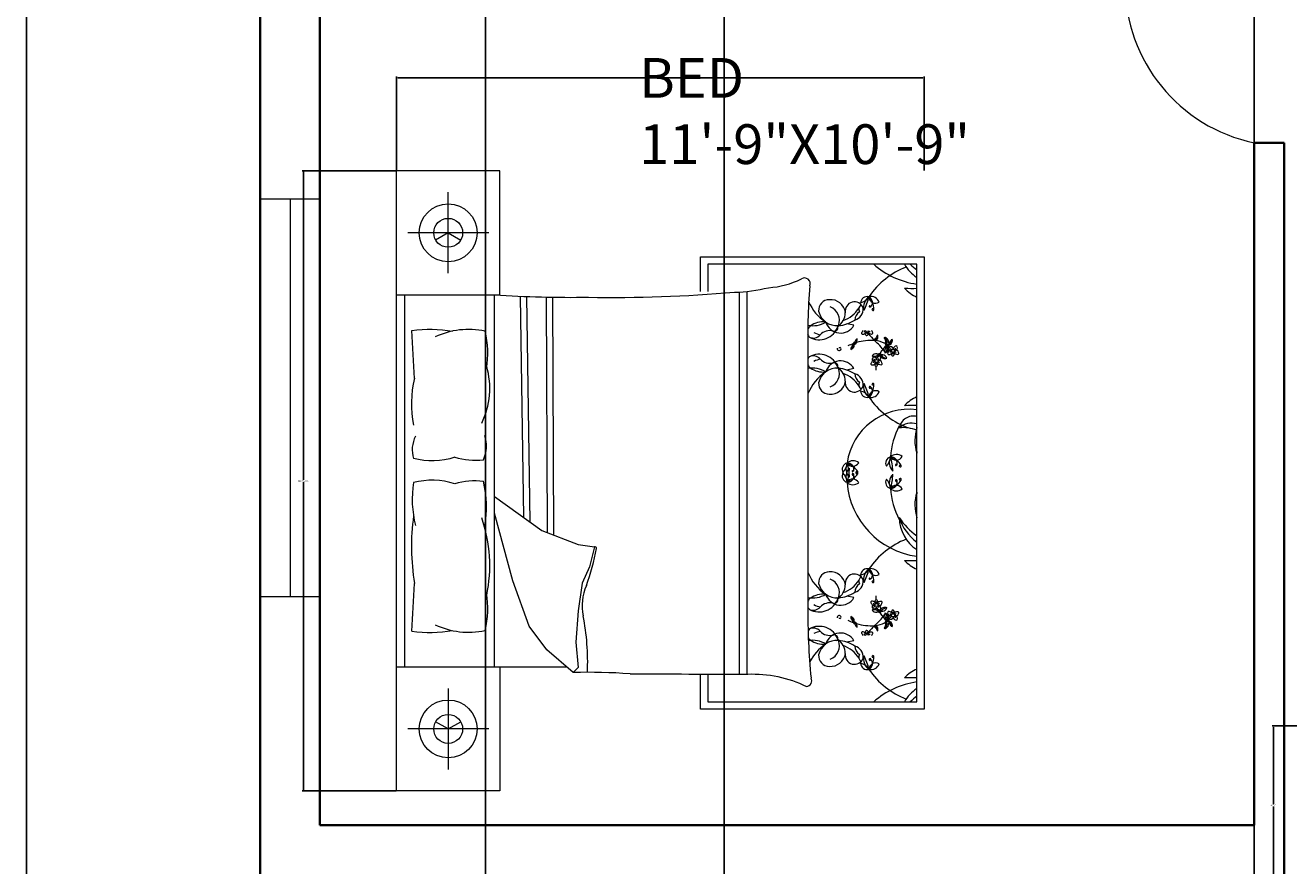
# Model space of a CAD drawing. Units: inches. Extents: x -59 to 444, y -680 to 63.
# Tile 4 of 9: x -59 to 132, y -270 to -143. Entities that reach past the tile are written whole.
import ezdxf

# ---------------------------------------------------------------- set-up
doc = ezdxf.new("R2010")
doc.units = ezdxf.units.IN
doc.header["$MEASUREMENT"] = 0
for name, color, linetype, lineweight in [('A-ANNO-DIMS', 2, 'Continuous', 18), ('A-AREA-IDEN', 7, 'Continuous', 18), ('A-DOOR', 3, 'Continuous', 18), ('A-FURN', 8, 'Continuous', 13), ('A-GLAZ', 4, 'Continuous', 18), ('A-WALL', 7, 'Continuous', 35)]:
    doc.layers.add(name, color=color, linetype=linetype, lineweight=lineweight)
doc.styles.get("Standard").update_dxf_attribs({"font": 'arial.ttf'})
doc.dimstyles.get("Standard").update_dxf_attribs({"dimtxt": 0.18, "dimasz": 0.18, "dimexe": 0.18, "dimexo": 0.0625, "dimgap": 0.09, "dimtad": 0, "dimtih": 1, "dimtoh": 1, "dimdec": 0, "dimzin": 0, "dimdsep": 46, "dimlunit": 3, "dimtxsty": 'Standard', "dimcen": 0.09, "dimadec": 0, "dimazin": 0, "dimtfac": 1, "dimtdec": 0, "dimtofl": 0, "dimtmove": 0, "dimatfit": 3, "dimfxl": 1, "dimtolj": 1, "dimtzin": 0, "dimarcsym": 0})

# ---------------------------------------------------------------- blocks, each defined once
blk = doc.blocks.new('BED-SET-80')
for p, q in [((0, 0), (0, 93.61)), ((7.8, 78.14), (7.8, 90.37)), ((13.92, 84.25), (1.69, 84.25)), ((45.89, 75.41), (45.89, 80.6)), ((45.89, 80.6), (79.61, 80.6)), ((79.61, 80.6), (79.61, 12.36)), ((46.97, 79.52), (46.97, 75.39)), ((78.53, 79.52), (46.97, 79.52)), ((78.53, 13.44), (78.53, 79.52)), ((1.2, 74.89), (1.2, 18.72)), ((14.79, 18.72), (14.79, 74.89)), ((18.68, 74.64), (19.15, 41.31)), ((19.64, 74.6), (20.12, 40.61)), ((22.59, 74.55), (22.73, 39.01)), ((23.55, 74.56), (23.7, 38.64)), ((51.73, 75.32), (51.73, 17.64)), ((52.89, 75.4), (52.89, 17.64)), ((69.04, 70.29), (67.98, 70.5)), ((62.09, 65.81), (62.09, 27.8)), ((69.04, 63.75), (67.98, 63.54)), ((14.79, 44.44), (21.93, 39.31)), ((17.58, 31.73), (14.79, 41.93)), ((21.93, 39.31), (27.43, 37.22)), ((27.43, 37.22), (29.89, 36.85)), ((29.89, 36.85), (29.13, 33.81)), ((29.13, 33.81), (28, 31.35)), ((20.04, 24.9), (17.58, 31.73)), ((28, 31.35), (27.43, 27.18)), ((69.04, 29.21), (67.98, 29.42)), ((27.43, 27.18), (27.05, 22.44)), ((22.69, 21.3), (20.04, 24.9)), ((26.67, 17.88), (22.69, 21.3)), ((27.05, 22.44), (27.43, 18.64)), ((69.04, 22.67), (67.98, 22.46)), ((0, 18.72), (25.69, 18.72)), ((27.43, 18.64), (26.67, 17.88)), ((45.89, 12.36), (45.89, 17.65)), ((46.97, 17.65), (46.97, 13.44)), ((7.8, 15.48), (7.8, 3.25)), ((46.97, 13.44), (78.53, 13.44)), ((79.61, 12.36), (45.89, 12.36)), ((13.92, 9.36), (1.69, 9.36))]:
    blk.add_line(p, q)
for points in [[(0, 74.89), (15.6, 74.89), (15.6, 93.61), (0, 93.61)], [(7.8, 84.25), (5.91, 83.16)], [(7.8, 84.25), (9.69, 83.16)], [(15.6, 18.72), (15.6, 0), (0, 0)], [(7.8, 9.36), (5.91, 10.45)], [(7.8, 9.36), (9.69, 10.45)]]:
    blk.add_lwpolyline(points)
for points in [[(50.99, 75.29, 0.056112), (56.14, 75.97, 0.095341), (61.1, 77.28)], [(2.33, 69.51, -0.074897), (8.45, 69.4, 0.472817)], [(8.79, 50.37, -0.14099), (2.55, 50.18, -0.235245)], [(8.79, 46.37, 0.14099), (2.55, 46.55, 0.235245)], [(2.33, 24.1, 0.074897), (8.45, 24.21, -0.472817)], [(35.24, 17.69, 0.001242), (53, 17.64, -0.127202), (61.86, 15.77)]]:
    blk.add_lwpolyline(points, format="xyb")
for centre, radius in [((7.8, 84.25), 4.37), ((7.8, 84.25), 2.18), ((72.43, 64.89), 0.238), ((74.94, 66.44), 0.238), ((72.43, 28.07), 0.238), ((74.94, 26.51), 0.238), ((7.8, 9.36), 4.37), ((7.8, 9.36), 2.18)]:
    blk.add_circle(centre, radius)
for centre, radius, start, end in [((81.38, 67.71), 12.22, 111.4092, 145.6135), ((80.17, 88.62), 12.22, 228.1144, 262.255), ((81.81, 82.49), 5.96, 209.8884, 236.5383), ((82.92, 84.63), 7.42, 223.5186, 233.6964), ((61.58, 76.58), 0.853, 336.5219, 123.8264), ((26.23, 242.71), 168.2, 266.1, 270.9282), ((32.35, 293.91), 219.42, 269.1145, 274.8735), ((153.14, 68.68), 91.09, 175.2402, 181.8035), ((71.05, 73.62), 1.01, 76.272, 177.0484), ((69.51, 75.7), 2.09, 284.7031, 328.6173), ((72.42, 73.04), 1.93, 125.7657, 194.5347), ((62.95, 76.46), 8.55, 332.8176, 347.4827), ((71.58, 73.28), 1.36, 20.9613, 102.2885), ((72.31, 74.64), 1.02, 181.7131, 301.5367), ((68.97, 72.57), 3.09, 2.0648, 41.1598), ((70.83, 73.72), 1, 316.2238, 62.3173), ((80.43, 79.15), 4.97, 221.0454, 247.4453), ((77.76, 92.77), 16.91, 266.3481, 272.5919), ((68.68, 76.7), 7.09, 203.6453, 236.3329), ((65.28, 72.57), 1.58, 88.9462, 185.5144), ((65.51, 71.92), 2.24, 7.1143, 95.0551), ((64.66, 71.04), 2.17, 338.5779, 68.4181), ((66.02, 75.22), 4.42, 288.2955, 328.7386), ((69.11, 72.43), 1.4, 19.1312, 189.736), ((68.69, 72.77), 1.75, 285.6955, 4.031), ((70.63, 72.72), 0.861, 126.7319, 206.0245), ((71.41, 73.14), 0.0797, 20.2667, 316.2271), ((71.9, 72.68), 0.152, 168.5166, 2.0648), ((71.83, 72.7), 0.0737, 52.0591, 168.5166), ((62.78, 74.1), 3.88, 259.249, 301.1782), ((64.47, 67.2), 3.61, 85.2696, 124.215), ((66.45, 73.05), 2.82, 193.079, 274.7067), ((67.02, 71.45), 2.33, 196.8663, 330.0915), ((65.01, 72.31), 2.72, 305.9599, 357.6409), ((66.37, 75.26), 5.02, 273.4924, 303.7117), ((71.02, 70.88), 1.87, 128.4175, 173.8338), ((-888.54, 17.91), 892.37, 2.85022, 3.31479), ((10.9, 57.59), 12.07, 78.2417, 114.8684), ((1.24, 66.17), 12.55, 348.9631, 14.8961), ((63.13, 69.29), 1.13, 127.675, 162.5814), ((63.13, 69.29), 1.13, 196.6343, 225.5483), ((63.79, 71.09), 2.98, 240.8249, 340.7178), ((62.9, 69.77), 1.4, 246.1646, 318.4347), ((64.33, 71.54), 2.69, 240.0851, 262.564), ((65.39, 67.57), 1.92, 74.8529, 138.4347), ((66.04, 69.98), 0.581, 254.8529, 12.6959), ((64.47, 67.2), 3.61, 53.6555, 57.2989), ((70.36, 69.11), 0.184, 125.0752, 284.7644), ((70.64, 69.18), 0.398, 127.3642, 168.4363), ((70.33, 69.5), 0.573, 277.4968, 341.2737), ((70.78, 69.23), 0.228, 88.1325, 178.8919), ((71.24, 68.99), 0.493, 136.3462, 189.6513), ((70.96, 68.94), 0.205, 189.6513, 312.3208), ((71.01, 69.51), 0.238, 183.2768, 356.7232), ((71.76, 69.08), 0.78, 164.2829, 186.9148), ((70.84, 69.08), 0.39, 312.3208, 40.2111), ((71.66, 69.52), 0.554, 201.6382, 274.947), ((70.93, 68.76), 0.724, 42.3896, 66.5724), ((78.23, 74.49), 8.89, 217.9541, 226.8459), ((71.45, 69.18), 0.394, 10.9597, 52.2379), ((71.69, 69.15), 0.183, 274.947, 37.5263), ((72.86, 68.35), 0.492, 115.5379, 168.6744), ((71.19, 69.05), 1.48, 329.344, 349.7412), ((70.01, 68.71), 2.64, 352.8698, 1.6736), ((66.92, 66.75), 0.18, 349.5616, 167.2949), ((71.63, 60.26), 7.75, 110.1059, 116.9968), ((67.62, 67.79), 1.48, 308.4388, 328.836), ((69.03, 66.66), 0.492, 129.5056, 182.6421), ((67.36, 69), 2.64, 296.5064, 305.3102), ((67.34, 67.64), 1.5, 336.3901, 344.4871), ((68.98, 67.25), 0.191, 83.9457, 185.6216), ((68.22, 67.43), 0.785, 328.836, 0.8141), ((68.62, 67.2), 0.449, 306.5232, 32.4668), ((69.16, 67.55), 0.191, 112.5583, 214.2343), ((69.03, 67.89), 0.449, 265.7131, 351.6568), ((68.64, 68.14), 0.785, 297.3659, 329.344), ((68.05, 68.81), 1.5, 313.6929, 321.7899), ((69.71, 67.79), 0.492, 115.5379, 168.6744), ((68.04, 68.49), 1.48, 329.344, 349.7412), ((71.63, 60.26), 7.75, 86.1723, 106.4158), ((66.86, 68.15), 2.64, 352.8698, 1.6736), ((72.31, 68.11), 0.191, 112.5583, 214.2343), ((72.18, 68.45), 0.449, 265.7131, 351.6568), ((71.79, 68.7), 0.785, 297.3659, 329.344), ((71.83, 64.13), 3.89, 60.7959, 85.244), ((63.55, 58.53), 12.79, 37.8256, 47.7588), ((71.2, 69.37), 1.5, 313.6929, 321.7899), ((76.99, 63.73), 4.66, 130.182, 149.456), ((73.72, 68.18), 0.266, 33.0979, 123.1364), ((67.86, 64.43), 6.96, 31.1156, 34.8118), ((73.34, 67.72), 0.721, 2.3172, 70.5201), ((74.42, 66.38), 0.769, 139.3812, 199.9959), ((72.99, 66.94), 1.09, 310.9365, 22.7695), ((73.93, 67.55), 0.208, 135.7354, 318.1297), ((73.58, 67.88), 0.276, 315.7354, 31.1156), ((73.35, 67.3), 0.64, 319.3812, 5.5456), ((74.09, 67.55), 0.208, 68.2452, 250.6395), ((73.61, 67.8), 0.621, 352.6008, 57.1845), ((75.83, 63.64), 4.15, 111.7087, 116.2181), ((71.83, 64.13), 3.89, 47.5083, 55.9967), ((74.2, 67.94), 0.621, 252.8042, 349.6943), ((73.61, 66.83), 0.661, 331.1838, 51.6792), ((74.27, 68), 0.276, 248.2452, 323.6254), ((74.02, 68.16), 0.721, 291.7087, 3.0299), ((74.52, 66.74), 0.234, 138.2946, 276.2474), ((74.61, 66.71), 0.325, 358.5719, 143.8954), ((68.88, 71.96), 6.96, 323.6254, 327.3216), ((74.59, 67.98), 0.266, 325.6077, 55.6462), ((75.66, 66.51), 0.752, 121.9501, 165.2442), ((75.12, 66.93), 0.47, 278.5614, 22.5914), ((75.39, 66.95), 0.236, 44.3732, 121.9501), ((63.13, 64.75), 1.13, 134.4517, 156.7144), ((63.79, 62.95), 2.98, 19.2822, 119.1751), ((62.9, 64.27), 1.4, 41.5653, 113.8354), ((64.33, 62.5), 2.69, 97.436, 119.9149), ((65.39, 66.48), 1.92, 221.5653, 285.1471), ((66.81, 66.77), 0.293, 169.5864, 349.5616), ((72.06, 64.56), 0.398, 93.635, 168.4363), ((72.07, 66.71), 1.09, 253.6301, 325.4631), ((72.38, 65.2), 0.769, 82.0748, 142.6895), ((72.29, 66.26), 0.79, 228.342, 274.9894), ((72.01, 65.18), 0.234, 138.2946, 276.2474), ((72.1, 65.15), 0.325, 358.5719, 143.8954), ((72.28, 65.4), 0.328, 208.8493, 269.9355), ((72.01, 65.33), 0.375, 274.2123, 318.1587), ((72.32, 66.13), 0.661, 273.8774, 357.1501), ((73.15, 64.95), 0.752, 121.9501, 165.2442), ((72.57, 66.6), 0.64, 262.0748, 308.2393), ((72.63, 65.24), 0.158, 262.868, 7.094), ((72.61, 65.37), 0.47, 278.5614, 22.5914), ((72.87, 64.56), 0.394, 10.9597, 118.7804), ((76.99, 63.73), 4.66, 156.1523, 156.9499), ((72.87, 65.39), 0.236, 44.3732, 121.9501), ((73.6, 65.94), 0.661, 181.4625, 249.4747), ((73.49, 66.46), 0.64, 215.1128, 261.2773), ((74, 66.43), 1.09, 197.889, 269.722), ((73.66, 66.06), 0.79, 248.3627, 295.0101), ((73.28, 65.07), 0.769, 20.6625, 81.2773), ((73.49, 66.88), 0.79, 285.6484, 332.2957), ((74.29, 66.04), 0.184, 125.0752, 284.7644), ((74.57, 66.11), 0.398, 93.635, 168.4363), ((74.26, 66.43), 0.573, 277.4968, 341.2737), ((74.71, 66.17), 0.228, 88.1325, 178.8919), ((74.8, 66.96), 0.328, 208.8493, 269.9355), ((74.52, 66.89), 0.375, 274.2123, 318.1587), ((75.17, 65.92), 0.493, 136.3462, 189.6513), ((74.89, 65.88), 0.205, 189.6513, 312.3208), ((75.68, 66.02), 0.78, 164.2829, 186.9148), ((74.76, 66.01), 0.39, 312.3208, 40.2111), ((75.59, 66.45), 0.554, 201.6382, 274.947), ((75.14, 66.8), 0.158, 262.868, 7.094), ((74.86, 65.69), 0.724, 42.3896, 66.5724), ((75.38, 66.12), 0.394, 10.9597, 118.7804), ((75.62, 66.08), 0.183, 274.947, 37.5263), ((2.16, 60.76), 11.92, 333.8761, 16.1746), ((63.13, 64.75), 1.13, 203.2856, 232.325), ((62.78, 59.95), 3.88, 58.8218, 100.2867), ((68.68, 57.35), 7.09, 123.6671, 158.5059), ((64.47, 66.84), 3.61, 235.785, 274.7304), ((66.45, 60.99), 2.82, 85.2933, 166.921), ((67.02, 62.59), 2.33, 29.9085, 163.1337), ((64.66, 63), 2.17, 291.5819, 21.4221), ((66.04, 64.06), 0.581, 347.3041, 105.1471), ((64.47, 66.84), 3.61, 302.7011, 306.3445), ((65.01, 61.74), 2.72, 2.3591, 54.0401), ((66.37, 58.78), 5.02, 56.2883, 86.5076), ((66.02, 58.82), 4.42, 31.2614, 71.7045), ((71.77, 64.48), 0.184, 125.0752, 284.7644), ((71.75, 64.87), 0.573, 277.4968, 341.2737), ((72.2, 64.61), 0.228, 88.1325, 178.8919), ((72.66, 64.37), 0.493, 136.3462, 189.6513), ((72.38, 64.32), 0.205, 189.6513, 312.3208), ((76.99, 63.73), 4.66, 175.2415, 182.8929), ((73.17, 64.46), 0.78, 164.2829, 186.9148), ((72.25, 64.45), 0.39, 312.3208, 40.2111), ((73.08, 64.89), 0.554, 201.6382, 274.947), ((72.34, 64.14), 0.724, 42.3896, 66.5724), ((73.11, 64.52), 0.183, 274.947, 37.5263), ((18.71, 58.4), 16.46, 166.3427, 191.1841), ((65.28, 61.48), 1.58, 174.4856, 271.0538), ((65.51, 62.12), 2.24, 264.9449, 352.8857), ((69.11, 61.61), 1.4, 170.264, 340.8688), ((71.02, 63.16), 1.87, 186.1662, 231.5825), ((68.69, 61.27), 1.75, 355.969, 74.3045), ((70.63, 61.32), 0.861, 153.9755, 233.2681), ((72.42, 61), 1.93, 165.4653, 234.2343), ((62.95, 57.58), 8.55, 12.5173, 27.1824), ((68.97, 61.47), 3.09, 318.8402, 357.9352), ((71.9, 61.36), 0.152, 357.9352, 191.4834), ((71.83, 61.35), 0.0737, 191.4834, 307.9409), ((71.05, 60.42), 1.01, 182.9516, 283.728), ((69.51, 58.35), 2.09, 31.3827, 75.2969), ((70.83, 60.32), 1, 297.6827, 43.7762), ((72.31, 59.4), 1.02, 58.4633, 178.2869), ((71.58, 60.76), 1.36, 257.7115, 339.0387), ((81.38, 66.34), 12.22, 214.3865, 248.5908), ((71.46, 60.92), 0.132, 43.7762, 339.7183), ((80.43, 54.89), 4.97, 112.5547, 138.9546), ((77.35, 48.15), 9.46, 82.8636, 171.8197), ((77.76, 41.28), 16.91, 87.4081, 93.6519), ((78.01, 54.39), 2.19, 76.3898, 169.0739), ((77.71, 52.75), 2.77, 72.8609, 131.9049), ((7, 51.46), 4.63, 153.3437, 196.1026), ((8.62, 52.09), 4.96, 335.0183, 18.5407), ((86.72, 49.48), 12.22, 152.5854, 175.5377), ((76.49, 49.37), 5.47, 68.117, 96.6195), ((84.95, 52.9), 6.72, 162.9798, 196.4569), ((11.92, 61.4), 11.47, 254.1707, 275.9871), ((68.9, 48.49), 1.36, 50.8855, 132.2127), ((74.82, 49.46), 1.01, 106.1963, 206.9726), ((72.45, 50.49), 2.09, 314.6273, 358.5415), ((76.29, 49.64), 1.93, 155.6899, 224.4589), ((75.44, 49.43), 1.36, 50.8855, 132.2127), ((75.4, 50.97), 1.02, 211.6373, 331.4609), ((73.53, 47.51), 3.09, 31.989, 71.0841), ((66.37, 47.87), 8.55, 2.7418, 17.407), ((74.57, 49.43), 1, 346.148, 92.2415), ((88.42, 50.24), 9.94, 174.3643, 175.6213), ((95.23, 45), 17.76, 160.0972, 160.2783), ((68.27, 48.52), 1.01, 106.1963, 206.9726), ((68.27, 47.56), 1.01, 153.0274, 253.8037), ((65.9, 49.55), 2.09, 314.6273, 358.5415), ((65.9, 46.53), 2.09, 1.4585, 45.3727), ((69.75, 48.7), 1.93, 155.6899, 224.4589), ((69.75, 47.38), 1.93, 135.5411, 204.3101), ((68.85, 50.03), 1.02, 211.6373, 331.4609), ((68.02, 48.5), 1, 346.148, 92.2415), ((66.98, 46.57), 3.09, 31.989, 71.0841), ((59.83, 46.94), 8.55, 2.7418, 17.407), ((59.83, 49.14), 8.55, 342.593, 357.2582), ((66.98, 49.51), 3.09, 288.9159, 328.011), ((68.02, 47.58), 1, 267.7585, 13.852), ((68.82, 48.28), 0.0797, 50.1909, 346.0209), ((68.87, 47.79), 0.132, 13.852, 309.9245), ((69.48, 48.13), 0.152, 198.4408, 31.989), ((69.4, 48.1), 0.0737, 81.9833, 198.4408), ((69.48, 47.95), 0.152, 328.011, 161.5592), ((69.4, 47.97), 0.0737, 161.5592, 278.0167), ((76.29, 46.44), 1.93, 135.5411, 204.3101), ((66.37, 48.21), 8.55, 342.593, 357.2582), ((75.36, 49.21), 0.0797, 50.1909, 346.0209), ((76.02, 49.07), 0.152, 198.4408, 31.989), ((75.95, 49.04), 0.0737, 81.9833, 198.4408), ((19.05, 44.1), 16.68, 171.5249, 193.96), ((11.92, 35.33), 11.47, 84.0129, 105.8293), ((-2.93, 42.85), 16.51, 349.8617, 13.6238), ((68.85, 46.05), 1.02, 28.5391, 148.3627), ((68.9, 47.59), 1.36, 227.7873, 309.1145), ((80.17, 47.53), 12.22, 184.4623, 262.255), ((74.82, 46.62), 1.01, 153.0274, 253.8037), ((72.45, 45.59), 2.09, 1.4585, 45.3727), ((73.53, 48.57), 3.09, 288.9159, 328.011), ((74.57, 46.65), 1, 267.7585, 13.852), ((75.4, 45.11), 1.02, 28.5391, 148.3627), ((75.41, 46.85), 0.132, 13.852, 309.9245), ((76.02, 47.01), 0.152, 328.011, 161.5592), ((75.95, 47.04), 0.0737, 161.5592, 278.0167), ((75.44, 46.65), 1.36, 227.7873, 309.1145), ((86.72, 46.6), 12.22, 184.4623, 207.4146), ((84.95, 43.18), 6.72, 163.5431, 197.0202), ((88.42, 45.84), 9.94, 184.3787, 185.6357), ((95.23, 51.08), 17.76, 199.7217, 199.9028), ((36.21, 36.93), 33.95, 172.2196, 189.497), ((-7.68, 34.04), 21.76, 348.0397, 19.2615), ((81.81, 41.4), 5.96, 181.272, 236.5383), ((85.01, 47.45), 11.04, 214.0123, 234.053), ((82.92, 43.54), 7.42, 197.8504, 233.6964), ((-5.48, 43.34), 36.3, 340.1194, 349.3383), ((29.97, 36.63), 0.226, 358.8623, 109.7536), ((81.38, 26.62), 12.22, 111.4092, 145.6135), ((77.76, 51.68), 16.91, 266.3481, 272.5919), ((80.43, 38.07), 4.97, 221.0454, 247.4453), ((68.68, 35.61), 7.09, 201.4941, 236.3329), ((65.28, 31.48), 1.58, 88.9462, 185.5144), ((65.51, 30.83), 2.24, 7.1143, 95.0551), ((69.11, 31.35), 1.4, 19.1312, 189.736), ((71.05, 32.54), 1.01, 76.272, 177.0484), ((69.51, 34.61), 2.09, 284.7031, 328.6173), ((72.42, 31.96), 1.93, 125.7657, 194.5347), ((62.95, 35.38), 8.55, 332.8176, 347.4827), ((71.58, 32.2), 1.36, 20.9613, 102.2885), ((70.83, 32.64), 1, 316.2238, 62.3173), ((68.97, 31.49), 3.09, 2.0648, 41.1598), ((72.31, 33.55), 1.02, 181.7131, 301.5367), ((-888.54, 75.7), 892.37, 356.68521, 357.14978), ((35.63, 27.93), 7.62, 156.2616, 191.3392), ((66.45, 31.97), 2.82, 193.079, 274.7067), ((64.66, 29.96), 2.17, 338.5779, 68.4181), ((65.01, 31.22), 2.72, 305.9599, 357.6409), ((66.02, 34.13), 4.42, 288.2955, 328.7386), ((68.69, 31.69), 1.75, 285.6955, 4.031), ((71.02, 29.8), 1.87, 128.4175, 173.8338), ((70.63, 31.64), 0.861, 126.7319, 206.0245), ((71.41, 32.05), 0.0797, 20.2667, 316.2271), ((71.9, 31.6), 0.152, 168.5166, 2.0648), ((71.83, 31.61), 0.0737, 52.0591, 168.5166), ((1.24, 27.44), 12.55, 345.1039, 11.0369), ((62.78, 33.01), 3.88, 259.7133, 301.1782), ((63.13, 28.21), 1.13, 127.675, 156.7144), ((63.79, 30.01), 2.98, 240.8249, 340.7178), ((64.47, 26.11), 3.61, 85.2696, 124.215), ((67.02, 30.37), 2.33, 196.8663, 330.0915), ((66.04, 28.9), 0.581, 254.8529, 12.6959), ((64.47, 26.11), 3.61, 53.6555, 57.2989), ((66.37, 34.18), 5.02, 273.4924, 303.7117), ((71.77, 28.47), 0.184, 75.2356, 234.9248), ((71.75, 28.08), 0.573, 18.7263, 82.5032), ((72.38, 28.64), 0.205, 47.6792, 170.3487), ((72.66, 28.59), 0.493, 170.3487, 223.6538), ((76.99, 29.23), 4.66, 177.1071, 184.7585), ((72.25, 28.51), 0.39, 319.7889, 47.6792), ((159.53, 26.69), 97.45, 179.3433, 185.6887), ((63.13, 28.21), 1.13, 203.229, 225.5483), ((62.9, 28.68), 1.4, 246.1646, 318.4347), ((64.33, 30.46), 2.69, 240.0851, 262.564), ((65.39, 26.48), 1.92, 74.8529, 138.4347), ((72.06, 28.4), 0.398, 191.5637, 266.365), ((72.01, 27.77), 0.234, 83.7526, 221.7054), ((72.29, 26.7), 0.79, 85.0106, 131.658), ((72.07, 26.25), 1.09, 34.5369, 106.3699), ((72.38, 27.76), 0.769, 217.3105, 277.9252), ((72.1, 27.81), 0.325, 216.1046, 1.4281), ((72.2, 28.35), 0.228, 181.1081, 271.8675), ((72.28, 27.56), 0.328, 90.0645, 151.1507), ((72.01, 27.63), 0.375, 41.8413, 85.7877), ((72.32, 26.83), 0.661, 2.8499, 86.1226), ((73.17, 28.5), 0.78, 173.0852, 195.7171), ((73.15, 28.01), 0.752, 194.7558, 238.0499), ((72.57, 26.36), 0.64, 51.7607, 97.9252), ((73.08, 28.07), 0.554, 85.053, 158.3618), ((72.63, 27.72), 0.158, 352.906, 97.132), ((72.34, 28.82), 0.724, 293.4276, 317.6104), ((72.87, 28.4), 0.394, 241.2196, 349.0403), ((72.61, 27.59), 0.47, 337.4086, 81.4386), ((76.99, 29.23), 4.66, 203.0501, 203.8477), ((72.87, 27.57), 0.236, 238.0499, 315.6268), ((73.6, 27.02), 0.661, 110.5253, 178.5375), ((74, 26.53), 1.09, 90.278, 162.111), ((73.49, 26.5), 0.64, 98.7227, 144.8872), ((76.99, 29.23), 4.66, 210.544, 229.818), ((73.11, 28.44), 0.183, 322.4737, 85.053), ((73.66, 26.9), 0.79, 64.9899, 111.6373), ((73.28, 27.89), 0.769, 278.7227, 339.3375), ((74.42, 26.58), 0.769, 160.0041, 220.6188), ((72.99, 26.02), 1.09, 337.2305, 49.0635), ((73.49, 26.08), 0.79, 27.7043, 74.3516), ((74.29, 26.92), 0.184, 75.2356, 234.9248), ((74.57, 26.84), 0.398, 191.5637, 266.365), ((74.26, 26.53), 0.573, 18.7263, 82.5032), ((74.71, 26.79), 0.228, 181.1081, 271.8675), ((75.17, 27.03), 0.493, 170.3487, 223.6538), ((74.89, 27.08), 0.205, 47.6792, 170.3487), ((75.68, 26.94), 0.78, 173.0852, 195.7171), ((74.76, 26.95), 0.39, 319.7889, 47.6792), ((75.59, 26.51), 0.554, 85.053, 158.3618), ((74.86, 27.26), 0.724, 293.4276, 317.6104), ((75.38, 26.84), 0.394, 241.2196, 349.0403), ((75.62, 26.88), 0.183, 322.4737, 85.053), ((10.9, 36.03), 12.07, 245.1316, 281.7583), ((-6.48, 19.49), 35.33, 357.4519, 11.3392), ((63.79, 21.87), 2.98, 19.2822, 119.1751), ((66.81, 26.19), 0.293, 10.4384, 190.4136), ((66.92, 26.21), 0.18, 192.7051, 10.4384), ((71.63, 32.69), 7.75, 243.0032, 249.8941), ((67.62, 25.17), 1.48, 31.164, 51.5612), ((69.03, 26.3), 0.492, 177.3579, 230.4944), ((67.36, 23.96), 2.64, 54.6898, 63.4936), ((67.34, 25.32), 1.5, 15.5129, 23.6099), ((68.98, 25.71), 0.191, 174.3784, 276.0543), ((68.62, 25.76), 0.449, 327.5332, 53.4768), ((68.22, 25.53), 0.785, 359.1859, 31.164), ((69.16, 25.41), 0.191, 145.7657, 247.4417), ((69.03, 25.07), 0.449, 8.3432, 94.2869), ((68.64, 24.82), 0.785, 30.656, 62.6341), ((68.05, 24.15), 1.5, 38.2101, 46.3071), ((69.71, 25.17), 0.492, 191.3256, 244.4621), ((68.04, 24.47), 1.48, 10.2588, 30.656), ((71.63, 32.69), 7.75, 253.5842, 273.8277), ((66.86, 24.81), 2.64, 358.3264, 7.1302), ((78.23, 18.47), 8.89, 133.1541, 142.0459), ((72.31, 24.85), 0.191, 145.7657, 247.4417), ((63.55, 34.43), 12.79, 312.2412, 322.1744), ((71.83, 28.83), 3.89, 274.756, 299.2041), ((72.18, 24.51), 0.449, 8.3432, 94.2869), ((71.79, 24.26), 0.785, 30.656, 62.6341), ((73.34, 25.24), 0.721, 289.4799, 357.6828), ((67.86, 28.53), 6.96, 325.1882, 328.8844), ((73.93, 25.41), 0.208, 41.8703, 224.2646), ((73.58, 25.08), 0.276, 328.8844, 44.2646), ((73.35, 25.66), 0.64, 354.4544, 40.6188), ((74.09, 25.41), 0.208, 109.3605, 291.7548), ((73.61, 25.16), 0.621, 302.8155, 7.3992), ((75.83, 29.32), 4.15, 243.7819, 248.2913), ((71.83, 28.83), 3.89, 304.0033, 312.4917), ((73.61, 26.13), 0.661, 308.3208, 28.8162), ((74.2, 25.02), 0.621, 10.3057, 107.1958), ((74.27, 24.96), 0.276, 36.3746, 111.7548), ((74.52, 26.22), 0.234, 83.7526, 221.7054), ((74.02, 24.8), 0.721, 356.9701, 68.2913), ((74.61, 26.25), 0.325, 216.1046, 1.4281), ((68.88, 21), 6.96, 32.6784, 36.3746), ((74.8, 26), 0.328, 90.0645, 151.1507), ((74.52, 26.07), 0.375, 41.8413, 85.7877), ((74.59, 24.98), 0.266, 304.3538, 34.3923), ((75.66, 26.45), 0.752, 194.7558, 238.0499), ((75.14, 26.16), 0.158, 352.906, 97.132), ((75.12, 26.03), 0.47, 337.4086, 81.4386), ((75.39, 26.01), 0.236, 238.0499, 315.6268), ((63.13, 23.67), 1.13, 134.4517, 153.558), ((63.13, 23.67), 1.13, 210.0293, 232.325), ((62.9, 23.19), 1.4, 41.5653, 113.8354), ((64.33, 21.42), 2.69, 97.436, 119.9149), ((65.39, 25.39), 1.92, 221.5653, 285.1471), ((67.02, 21.51), 2.33, 29.9085, 163.1337), ((66.04, 22.98), 0.581, 347.3041, 105.1471), ((70.36, 23.85), 0.184, 75.2356, 234.9248), ((70.64, 23.78), 0.398, 191.5637, 232.6358), ((70.33, 23.46), 0.573, 18.7263, 82.5032), ((70.78, 23.73), 0.228, 181.1081, 271.8675), ((71.24, 23.97), 0.493, 170.3487, 223.6538), ((70.96, 24.02), 0.205, 47.6792, 170.3487), ((71.01, 23.45), 0.238, 3.2768, 176.7232), ((71.76, 23.88), 0.78, 173.0852, 195.7171), ((70.84, 23.88), 0.39, 319.7889, 47.6792), ((71.66, 23.44), 0.554, 85.053, 158.3618), ((70.93, 24.2), 0.724, 293.4276, 317.6104), ((71.45, 23.78), 0.394, 307.7621, 349.0403), ((71.69, 23.81), 0.183, 322.4737, 85.053), ((71.2, 23.59), 1.5, 38.2101, 46.3071), ((72.86, 24.61), 0.492, 191.3256, 244.4621), ((71.19, 23.91), 1.48, 10.2588, 30.656), ((70.01, 24.25), 2.64, 358.3264, 7.1302), ((73.72, 24.78), 0.266, 236.8636, 326.9021), ((62.78, 18.86), 3.88, 58.8218, 99.1554), ((68.68, 16.26), 7.09, 123.6671, 153.2997), ((64.47, 25.76), 3.61, 235.785, 274.7304), ((66.45, 19.91), 2.82, 85.2933, 166.921), ((64.66, 21.92), 2.17, 291.5819, 21.4221), ((64.47, 25.76), 3.61, 302.7011, 306.3445), ((65.01, 20.65), 2.72, 2.3591, 54.0401), ((66.37, 17.7), 5.02, 56.2883, 86.5076), ((66.02, 17.74), 4.42, 31.2614, 71.7045), ((68.69, 20.19), 1.75, 355.969, 74.3045), ((71.02, 22.08), 1.87, 186.1662, 231.5825), ((65.28, 20.39), 1.58, 174.4856, 271.0538), ((65.51, 21.04), 2.24, 264.9449, 352.8857), ((69.11, 20.52), 1.4, 170.264, 340.8688), ((70.63, 20.24), 0.861, 153.9755, 233.2681), ((69.51, 17.26), 2.09, 31.3827, 75.2969), ((71.05, 19.33), 1.01, 182.9516, 283.728), ((72.42, 19.92), 1.93, 165.4653, 234.2343), ((62.95, 16.5), 8.55, 12.5173, 27.1824), ((68.97, 20.38), 3.09, 318.8402, 357.9352), ((70.83, 19.24), 1, 297.6827, 43.7762), ((72.31, 18.32), 1.02, 58.4633, 178.2869), ((71.58, 19.67), 1.36, 257.7115, 339.0387), ((71.46, 19.84), 0.132, 43.7762, 339.7183), ((71.9, 20.28), 0.152, 357.9352, 191.4834), ((71.83, 20.26), 0.0737, 191.4834, 307.9409), ((29, -67.95), 85.86, 85.8294, 91.553), ((81.38, 25.25), 12.22, 214.3865, 248.5908), ((80.43, 13.81), 4.97, 112.5547, 138.9546), ((61.8, 16.63), 0.864, 273.98, 27.3412), ((80.17, 4.34), 12.22, 97.745, 131.8856), ((81.81, 10.47), 5.96, 123.4617, 150.1116), ((77.76, 0.19), 16.91, 87.4081, 93.6519), ((82.92, 8.33), 7.42, 126.3036, 136.4814)]:
    blk.add_arc(centre, radius, start, end)
blk = doc.blocks.new('WIN-60-W9')
for p, q in [((60, 9), (0, 9)), ((0, 9), (0, 0)), ((60, 0), (60, 9)), ((0, 4.5), (60, 4.5)), ((0, 0), (60, 0))]:
    blk.add_line(p, q)
blk = doc.blocks.new('*D17')
at = {"layer": 'A-ANNO-DIMS', "color": 0, "lineweight": -2, "transparency": 16777216}
for p, q in [((133.17, -248.44), (129.45, -248.44)), ((129.63, -248.62), (129.63, -260.25)), ((129.63, -272.26), (129.63, -260.62)), ((133.17, -272.44), (129.45, -272.44))]:
    blk.add_line(p, q, dxfattribs=at)
at = {"layer": 'A-ANNO-DIMS', "color": 0, "transparency": 16777216}
for points in [[(129.6, -248.62), (129.66, -248.62), (129.63, -248.44)], [(129.6, -272.26), (129.66, -272.26), (129.63, -272.44)]]:
    blk.add_solid(points, dxfattribs=at)
at = {"layer": 'Defpoints', "color": 0, "transparency": 16777216}
for p in [(133.23, -248.44), (129.63, -272.44), (133.23, -272.44)]:
    blk.add_point(p, dxfattribs=at)
at = {"layer": 'A-ANNO-DIMS', "color": 0, "transparency": 16777216, "insert": (129.63, -260.44), "char_height": 0.18, "attachment_point": 5}
blk.add_mtext('\\A1;24 TYP.', dxfattribs=at)
blk = doc.blocks.new('*D36')
at = {"layer": 'A-ANNO-DIMS', "color": 0, "lineweight": -2, "transparency": 16777216}
for p, q in [((-2.77, -164.66), (-16.93, -164.66)), ((-16.75, -164.84), (-16.75, -211.29)), ((-16.75, -258.09), (-16.75, -211.65)), ((-2.77, -258.27), (-16.93, -258.27))]:
    blk.add_line(p, q, dxfattribs=at)
at = {"layer": 'A-ANNO-DIMS', "color": 0, "transparency": 16777216}
for points in [[(-16.78, -164.84), (-16.72, -164.84), (-16.75, -164.66)], [(-16.78, -258.09), (-16.72, -258.09), (-16.75, -258.27)]]:
    blk.add_solid(points, dxfattribs=at)
at = {"layer": 'Defpoints', "color": 0, "transparency": 16777216}
for p in [(-16.75, -164.66), (-2.71, -164.66), (-2.71, -258.27)]:
    blk.add_point(p, dxfattribs=at)
at = {"layer": 'A-ANNO-DIMS', "color": 0, "transparency": 16777216, "insert": (-16.75, -211.47), "char_height": 0.18, "attachment_point": 5}
blk.add_mtext('\\A1;BED B 94 TYP.', dxfattribs=at)
blk = doc.blocks.new('*D37')
at = {"layer": 'A-ANNO-DIMS', "color": 0, "lineweight": -2, "transparency": 16777216}
for p, q in [((-2.71, -164.6), (-2.71, -150.44)), ((-2.53, -150.62), (36.57, -150.62)), ((76.72, -150.62), (37.63, -150.62)), ((76.9, -164.6), (76.9, -150.44))]:
    blk.add_line(p, q, dxfattribs=at)
at = {"layer": 'A-ANNO-DIMS', "color": 0, "transparency": 16777216}
for points in [[(-2.53, -150.59), (-2.53, -150.65), (-2.71, -150.62)], [(76.72, -150.59), (76.72, -150.65), (76.9, -150.62)]]:
    blk.add_solid(points, dxfattribs=at)
at = {"layer": 'Defpoints', "color": 0, "transparency": 16777216}
for p in [(76.9, -150.62), (-2.71, -164.66), (76.9, -164.66)]:
    blk.add_point(p, dxfattribs=at)
at = {"layer": 'A-ANNO-DIMS', "color": 0, "transparency": 16777216, "insert": (37.1, -150.62), "char_height": 0.18, "attachment_point": 5}
blk.add_mtext('\\A1;80 TYP.', dxfattribs=at)
blk = doc.blocks.new('*D48')
at = {"layer": 'A-ANNO-DIMS', "color": 0, "lineweight": -2, "transparency": 16777216}
for p, q in [((-23.33, 15.56), (-58.7, 15.56)), ((-58.52, 15.38), (-58.52, -128.25)), ((-58.52, -272.26), (-58.52, -128.62)), ((-23.33, -272.44), (-58.7, -272.44))]:
    blk.add_line(p, q, dxfattribs=at)
at = {"layer": 'A-ANNO-DIMS', "color": 0, "transparency": 16777216}
for points in [[(-58.55, 15.38), (-58.49, 15.38), (-58.52, 15.56)], [(-58.55, -272.26), (-58.49, -272.26), (-58.52, -272.44)]]:
    blk.add_solid(points, dxfattribs=at)
at = {"layer": 'Defpoints', "color": 0, "transparency": 16777216}
for p in [(-23.27, 15.56), (-58.52, -272.44), (-23.27, -272.44)]:
    blk.add_point(p, dxfattribs=at)
at = {"layer": 'A-ANNO-DIMS', "color": 0, "transparency": 16777216, "insert": (-58.52, -128.44), "char_height": 0.18, "attachment_point": 5}
blk.add_mtext('\\A1;288', dxfattribs=at)
blk = doc.blocks.new('*D54')
at = {"layer": 'A-ANNO-DIMS', "color": 0, "lineweight": -2, "transparency": 16777216}
for p, q in [((10.73, -344.37), (10.73, 62.74)), ((10.91, 62.56), (28.51, 62.56)), ((46.55, 62.56), (28.95, 62.56)), ((46.73, -344.37), (46.73, 62.74))]:
    blk.add_line(p, q, dxfattribs=at)
at = {"layer": 'A-ANNO-DIMS', "color": 0, "transparency": 16777216}
for points in [[(10.91, 62.59), (10.91, 62.53), (10.73, 62.56)], [(46.55, 62.59), (46.55, 62.53), (46.73, 62.56)]]:
    blk.add_solid(points, dxfattribs=at)
at = {"layer": 'Defpoints', "color": 0, "transparency": 16777216}
for p in [(46.73, 62.56), (10.73, -344.44), (46.73, -344.44)]:
    blk.add_point(p, dxfattribs=at)
at = {"layer": 'A-ANNO-DIMS', "color": 0, "transparency": 16777216, "insert": (28.73, 62.56), "char_height": 0.18, "attachment_point": 5}
blk.add_mtext('\\A1;36', dxfattribs=at)
blk = doc.blocks.new('*D55')
at = {"layer": 'A-ANNO-DIMS', "color": 0, "lineweight": -2, "transparency": 16777216}
for p, q in [((46.73, -344.37), (46.73, 62.74)), ((46.91, 62.56), (86.51, 62.56)), ((126.55, 62.56), (86.95, 62.56)), ((126.73, -344.37), (126.73, 62.74))]:
    blk.add_line(p, q, dxfattribs=at)
at = {"layer": 'A-ANNO-DIMS', "color": 0, "transparency": 16777216}
for points in [[(46.91, 62.59), (46.91, 62.53), (46.73, 62.56)], [(126.55, 62.59), (126.55, 62.53), (126.73, 62.56)]]:
    blk.add_solid(points, dxfattribs=at)
at = {"layer": 'Defpoints', "color": 0, "transparency": 16777216}
for p in [(126.73, 62.56), (46.73, -344.44), (126.73, -344.44)]:
    blk.add_point(p, dxfattribs=at)
at = {"layer": 'A-ANNO-DIMS', "color": 0, "transparency": 16777216, "insert": (86.73, 62.56), "char_height": 0.18, "attachment_point": 5}
blk.add_mtext('\\A1;80', dxfattribs=at)
blk = doc.blocks.new('*D56')
at = {"layer": 'A-ANNO-DIMS', "color": 0, "lineweight": -2, "transparency": 16777216}
for p, q in [((126.73, -344.37), (126.73, 62.74)), ((126.91, 62.56), (158.65, 62.56)), ((191.05, 62.56), (159.3, 62.56)), ((191.23, -344.37), (191.23, 62.74))]:
    blk.add_line(p, q, dxfattribs=at)
at = {"layer": 'A-ANNO-DIMS', "color": 0, "transparency": 16777216}
for points in [[(126.91, 62.59), (126.91, 62.53), (126.73, 62.56)], [(191.05, 62.59), (191.05, 62.53), (191.23, 62.56)]]:
    blk.add_solid(points, dxfattribs=at)
at = {"layer": 'Defpoints', "color": 0, "transparency": 16777216}
for p in [(191.23, 62.56), (126.73, -344.44), (191.23, -344.44)]:
    blk.add_point(p, dxfattribs=at)
at = {"layer": 'A-ANNO-DIMS', "color": 0, "transparency": 16777216, "insert": (158.98, 62.56), "char_height": 0.18, "attachment_point": 5}
blk.add_mtext('\\A1;64.5', dxfattribs=at)

msp = doc.modelspace()

# ---------------------------------------------------------------- linework, layer by layer
at = {"layer": 'A-DOOR'}
msp.add_arc((131.75, -136.44), 24.52, 180, 258.1877, dxfattribs=at)
at = {"layer": 'A-WALL'}
for p, q in [((-23.27, 15.56), (-23.27, -272.44)), ((-14.27, -134.44), (-14.27, -263.44)), ((131.23, -160.44), (126.73, -160.44)), ((126.73, -160.44), (126.73, -263.44)), ((131.23, -160.44), (131.23, -272.44)), ((-14.27, -263.44), (126.73, -263.44))]:
    msp.add_line(p, q, dxfattribs=at)

# ---------------------------------------------------------------- block references
at = {"layer": 'A-FURN'}
msp.add_blockref('BED-SET-80', (-2.71, -258.27), dxfattribs=at)
at = {"layer": 'A-GLAZ', "rotation": 270.0000000000001}
msp.add_blockref('WIN-60-W9', (-23.27, -168.93), dxfattribs=at)

# ---------------------------------------------------------------- texts
at = {"layer": 'A-AREA-IDEN', "insert": (33.91, -147.64), "char_height": 6, "attachment_point": 1}
msp.add_mtext('BED\\P11\'-9"X10\'-9"', dxfattribs=at)

# ---------------------------------------------------------------- dimensions: what is measured, and where the dimension line sits
at = {"layer": 'A-ANNO-DIMS'}
for base, p1, p2, override, picture, middle in [((46.73, 62.56), (10.73, -344.44), (46.73, -344.44), {"dimdec": 0, "dimlfac": 1, "dimrnd": 0, "dimzin": 0, "dimdsep": 46, "dimlunit": 2}, '*D54', (28.73, 62.56)), ((126.73, 62.56), (46.73, -344.44), (126.73, -344.44), {"dimdec": 0, "dimlfac": 1, "dimrnd": 0, "dimzin": 0, "dimdsep": 46, "dimlunit": 2}, '*D55', (86.73, 62.56)), ((191.23, 62.56), (126.73, -344.44), (191.23, -344.44), {"dimdec": 1, "dimlfac": 1, "dimrnd": 0, "dimzin": 0, "dimdsep": 46, "dimlunit": 2}, '*D56', (158.98, 62.56))]:
    dim = msp.add_linear_dim(base=base, p1=p1, p2=p2, dimstyle='Standard', override=override, dxfattribs=at)
    dim.commit()
    dim.dimension.update_dxf_attribs({"geometry": picture, "text_midpoint": middle})
dim = msp.add_linear_dim(base=(-58.52, -272.44), p1=(-23.27, 15.56), p2=(-23.27, -272.44), angle=90, dimstyle='Standard', override={"dimdec": 0, "dimlfac": 1, "dimrnd": 0, "dimzin": 0, "dimdsep": 46, "dimlunit": 2}, dxfattribs=at)
dim.commit()
dim.dimension.update_dxf_attribs({"geometry": '*D48', "text_midpoint": (-58.52, -128.44)})
dim = msp.add_linear_dim(base=(76.9, -150.62), p1=(-2.71, -164.66), p2=(76.9, -164.66), text='<> TYP.', dimstyle='Standard', override={"dimdec": 0, "dimlfac": 1, "dimrnd": 0, "dimzin": 0, "dimdsep": 46, "dimlunit": 2}, dxfattribs=at)
dim.commit()
dim.dimension.update_dxf_attribs({"geometry": '*D37', "text_midpoint": (37.1, -150.62)})
for base, p1, p2, angle, text, picture, middle in [((-16.75, -164.66), (-2.71, -258.27), (-2.71, -164.66), 90, 'BED B <> TYP.', '*D36', (-16.75, -211.47)), ((129.63, -272.44), (133.23, -248.44), (133.23, -272.44), 270, '<> TYP.', '*D17', (129.63, -260.44))]:
    dim = msp.add_linear_dim(base=base, p1=p1, p2=p2, angle=angle, text=text, dimstyle='Standard', override={"dimdec": 0, "dimlfac": 1, "dimrnd": 0, "dimzin": 0, "dimdsep": 46, "dimlunit": 2}, dxfattribs=at)
    dim.commit()
    dim.dimension.update_dxf_attribs({"geometry": picture, "text_midpoint": middle})

doc.saveas('drawing.dxf')
